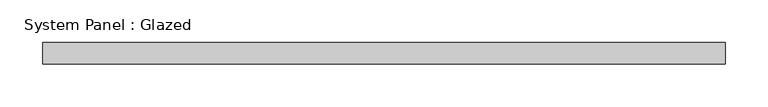
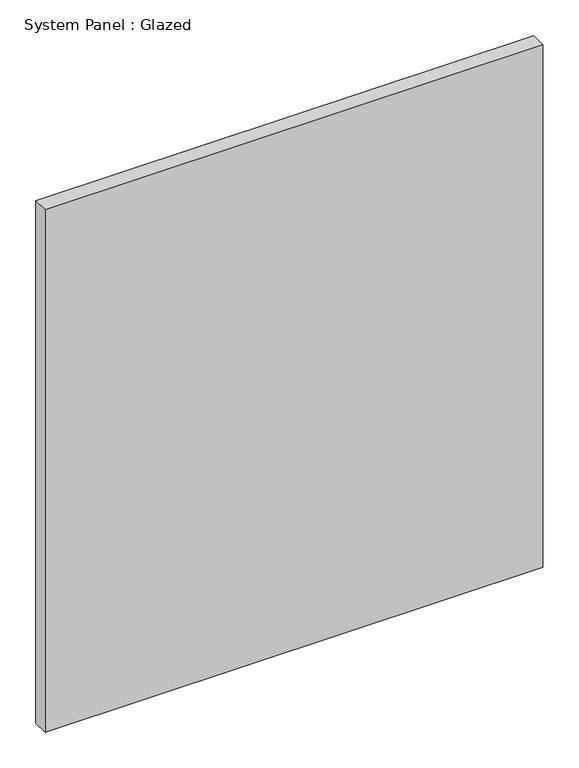
"""IFC4 building model written with IfcOpenShell, lengths in millimetres: plate geometry, System Panel : Glazed."""

from ifc_helpers import new_model, si_unit, origin, origin_with_axes, place, context, project, spatial, polyline, outline, extrude, source, transform, mapped, element, save


def system_panel_glazed_5de3b49f(model_context):
    return source(origin(), model_context, "Body", "SweptSolid", [
        extrude(outline(polyline([(400.05, 19.05), (-400.05, 19.05), (-400.05, 44.45), (400.05, 44.45), (400.05, 19.05)])), origin_with_axes(), (0.0, 0.0, 1.0), 887.8244987),
    ])


if __name__ == "__main__":
    model = new_model("IFC4")
    model_context = context("Model", 3, world=origin())
    ifc_project = project(units=[si_unit("LENGTHUNIT", "METRE", prefix="MILLI")], contexts=[model_context])
    site = spatial("IfcSite", under=ifc_project)
    building = spatial("IfcBuilding", under=site)
    placement = place(None, origin())
    system_panel_glazed_shape = system_panel_glazed_5de3b49f(model_context)
    element("IfcPlate", 1, ObjectType="System Panel : Glazed", at=placement, inside=building, context=model_context, shape_type="MappedRepresentation", body=[
        mapped(system_panel_glazed_shape, transform((0.0, 0.0, 0.0), x_axis=(1.0, 0.0, 0.0), y_axis=(0.0, 1.0, 0.0), z_axis=(0.0, 0.0, 1.0))),
    ])
    save(model, "model.ifc")

# Revit data of these elements
# Type "System Panel : Glazed"
#   Construction Type Id = "GSP4R"
#   Analytic Construction = "1/8 in Pilkington single glazing"
#   Visual Light Transmittance = 0.9
#   Solar Heat Gain Coefficient = 0.86
#   Heat Transfer Coefficient (U) = 1.18115 BTU/(h·ft²·°F)
#   Define Thermal Properties by = 1
# Element 1 (IfcPlate, "System Panel : Glazed")
#   Materials on its faces: "Glass"
# Materials
#   "Glass": class "Glass", colour RGB 0 128 192, transparency 0.75, Description = "Soda Lime Glass", Cost = 0
